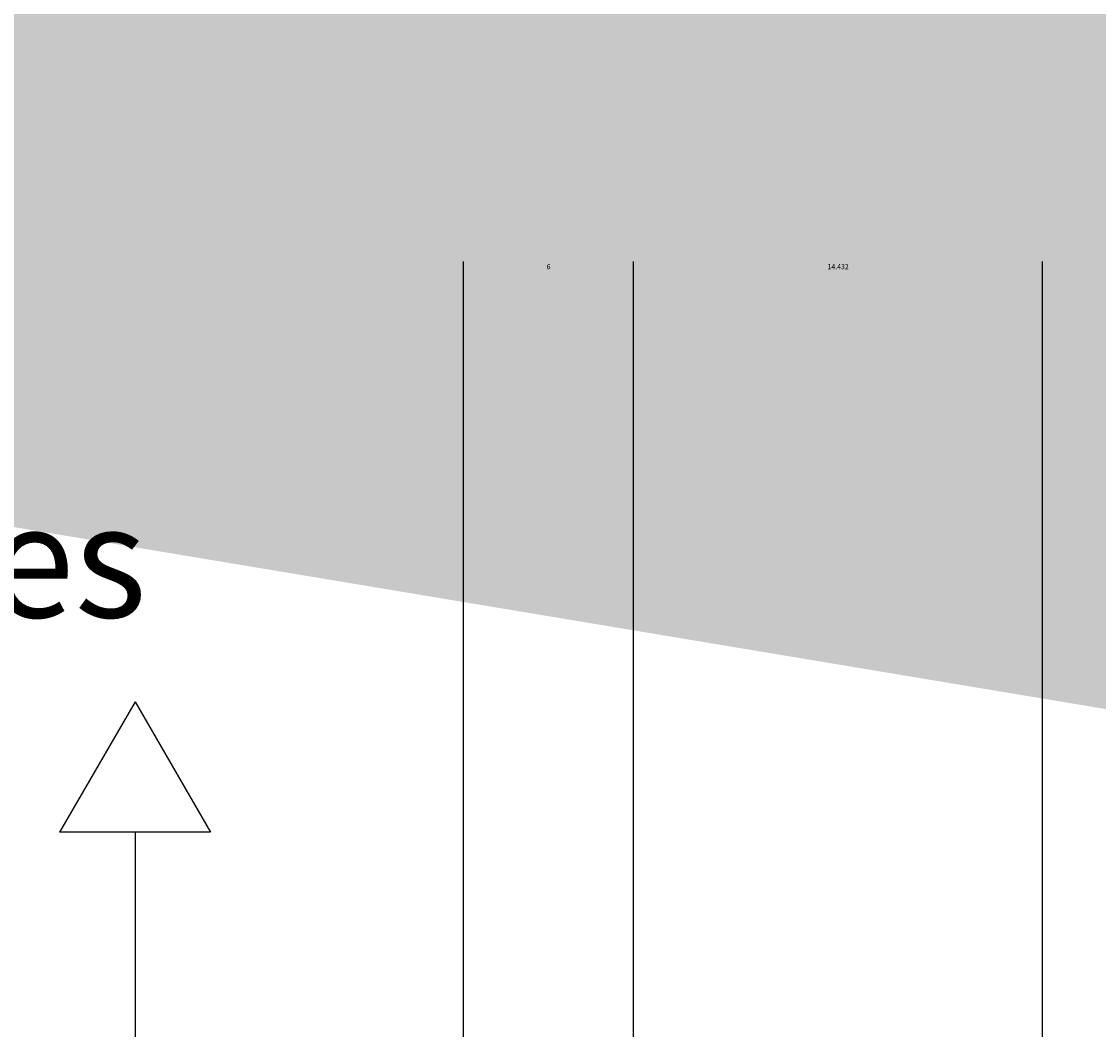
# Model space of a CAD drawing. Units: millimetres. Extents: x -22994 to 29398, y -19990 to 20176.
# Tile 113 of 135: x 166 to 204, y 177 to 213. Entities that reach past the tile are written whole.
import ezdxf

# ---------------------------------------------------------------- set-up
doc = ezdxf.new("R2010")
doc.units = ezdxf.units.MM
doc.header["$MEASUREMENT"] = 0
for name, color, linetype, lineweight in [('M-ANNO-SYMB', 7, 'Continuous', 25), ('M-ANNO-TEXT', 7, 'Continuous', 25), ('M-DIMS', 2, 'Continuous', 18)]:
    doc.layers.add(name, color=color, linetype=linetype, lineweight=lineweight)
doc.styles.get("Standard").update_dxf_attribs({"font": 'arial.ttf'})
doc.dimstyles.get("Standard").update_dxf_attribs({"dimtxt": 0.18, "dimasz": 10000, "dimexe": 0.18, "dimexo": 0.0625, "dimgap": 0.09, "dimtad": 0, "dimtih": 1, "dimtoh": 1, "dimdec": 0, "dimzin": 0, "dimdsep": 46, "dimtxsty": 'Standard', "dimcen": 0.09, "dimadec": 0, "dimazin": 0, "dimtfac": 1, "dimtdec": 0, "dimtofl": 0, "dimtmove": 0, "dimatfit": 3, "dimfxl": 1, "dimtolj": 1, "dimtzin": 0, "dimlwd": 30, "dimarcsym": 0})

# ---------------------------------------------------------------- blocks, each defined once
blk = doc.blocks.new('ARROW-FLOW')
for p, q in [((4.609, 5.322), (0, 2.661)), ((4.609, 5.322), (4.609, 0)), ((4.609, 0), (0, 2.661))]:
    blk.add_line(p, q)
blk = doc.blocks.new('*D2')
at = {"layer": 'Defpoints', "color": 0, "transparency": 16777216}
for p in [(6.677, 10.271), (290.852, 10.271), (290.852, -5.079)]:
    blk.add_point(p, dxfattribs=at)
at = {"layer": 'M-DIMS', "color": 0, "lineweight": -2, "transparency": 16777216}
for p, q in [((6.677, 10.209), (6.677, -5.259)), ((290.852, 10.209), (290.852, -5.259))]:
    blk.add_line(p, q, dxfattribs=at)
at = {"layer": 'M-DIMS', "color": 0, "lineweight": 30, "transparency": 16777216}
for p, q in [((-9993.323, -5.079), (-19993.323, -5.079)), ((10290.852, -5.079), (20290.852, -5.079))]:
    blk.add_line(p, q, dxfattribs=at)
at = {"layer": 'M-DIMS', "color": 0, "transparency": 16777216}
for points in [[(-9993.323, 1661.588), (-9993.323, -1671.745), (6.677, -5.079)], [(10290.852, 1661.588), (10290.852, -1671.745), (290.852, -5.079)]]:
    blk.add_solid(points, dxfattribs=at)
at = {"layer": 'M-DIMS', "color": 0, "transparency": 16777216, "insert": (148.765, -5.079), "char_height": 0.18, "attachment_point": 5}
blk.add_mtext('\\A1;284.2', dxfattribs=at)
blk = doc.blocks.new('*D3')
at = {"layer": 'Defpoints', "color": 0, "transparency": 16777216}
for p in [(110.265, 204.165), (110.265, 176.366), (95.833, 127.967)]:
    blk.add_point(p, dxfattribs=at)
at = {"layer": 'M-DIMS', "color": 0, "lineweight": 30, "transparency": 16777216}
for p, q in [((-9904.167, 204.165), (-19904.167, 204.165)), ((10110.265, 204.165), (20110.265, 204.165))]:
    blk.add_line(p, q, dxfattribs=at)
at = {"layer": 'M-DIMS', "color": 0, "lineweight": -2, "transparency": 16777216}
for p, q in [((95.833, 128.03), (95.833, 204.345)), ((110.265, 176.429), (110.265, 204.345))]:
    blk.add_line(p, q, dxfattribs=at)
at = {"layer": 'M-DIMS', "color": 0, "transparency": 16777216}
for points in [[(-9904.167, 1870.832), (-9904.167, -1462.501), (95.833, 204.165)], [(10110.265, 1870.832), (10110.265, -1462.501), (110.265, 204.165)]]:
    blk.add_solid(points, dxfattribs=at)
at = {"layer": 'M-DIMS', "color": 0, "transparency": 16777216, "insert": (103.049, 204.165), "char_height": 0.18, "attachment_point": 5}
blk.add_mtext('\\A1;14.432', dxfattribs=at)
blk = doc.blocks.new('*D4')
at = {"layer": 'Defpoints', "color": 0, "transparency": 16777216}
for p in [(116.265, 204.165), (110.265, 176.366), (116.265, 176.366)]:
    blk.add_point(p, dxfattribs=at)
at = {"layer": 'M-DIMS', "color": 0, "lineweight": 30, "transparency": 16777216}
for p, q in [((-9889.735, 204.165), (-19889.735, 204.165)), ((10116.265, 204.165), (20116.265, 204.165))]:
    blk.add_line(p, q, dxfattribs=at)
at = {"layer": 'M-DIMS', "color": 0, "lineweight": -2, "transparency": 16777216}
for p, q in [((110.265, 176.429), (110.265, 204.345)), ((116.265, 176.429), (116.265, 204.345))]:
    blk.add_line(p, q, dxfattribs=at)
at = {"layer": 'M-DIMS', "color": 0, "transparency": 16777216}
for points in [[(-9889.735, 1870.832), (-9889.735, -1462.501), (110.265, 204.165)], [(10116.265, 1870.832), (10116.265, -1462.501), (116.265, 204.165)]]:
    blk.add_solid(points, dxfattribs=at)
at = {"layer": 'M-DIMS', "color": 0, "transparency": 16777216, "insert": (113.265, 204.165), "char_height": 0.18, "attachment_point": 5}
blk.add_mtext('\\A1;6', dxfattribs=at)
blk = doc.blocks.new('*D5')
at = {"layer": 'Defpoints', "color": 0, "transparency": 16777216}
for p in [(181.265, 204.165), (116.265, 176.366), (181.265, 176.366)]:
    blk.add_point(p, dxfattribs=at)
at = {"layer": 'M-DIMS', "color": 0, "lineweight": 30, "transparency": 16777216}
for p, q in [((-9883.735, 204.165), (-19883.735, 204.165)), ((10181.265, 204.165), (20181.265, 204.165))]:
    blk.add_line(p, q, dxfattribs=at)
at = {"layer": 'M-DIMS', "color": 0, "lineweight": -2, "transparency": 16777216}
for p, q in [((116.265, 176.429), (116.265, 204.345)), ((181.265, 176.429), (181.265, 204.345))]:
    blk.add_line(p, q, dxfattribs=at)
at = {"layer": 'M-DIMS', "color": 0, "transparency": 16777216}
for points in [[(-9883.735, 1870.832), (-9883.735, -1462.501), (116.265, 204.165)], [(10181.265, 1870.832), (10181.265, -1462.501), (181.265, 204.165)]]:
    blk.add_solid(points, dxfattribs=at)
at = {"layer": 'M-DIMS', "color": 0, "transparency": 16777216, "insert": (148.765, 204.165), "char_height": 0.18, "attachment_point": 5}
blk.add_mtext('\\A1;65', dxfattribs=at)
blk = doc.blocks.new('*D6')
at = {"layer": 'Defpoints', "color": 0, "transparency": 16777216}
for p in [(187.265, 204.165), (181.265, 176.366), (187.265, 176.366)]:
    blk.add_point(p, dxfattribs=at)
at = {"layer": 'M-DIMS', "color": 0, "lineweight": 30, "transparency": 16777216}
for p, q in [((-9818.735, 204.165), (-19818.735, 204.165)), ((10187.265, 204.165), (20187.265, 204.165))]:
    blk.add_line(p, q, dxfattribs=at)
at = {"layer": 'M-DIMS', "color": 0, "lineweight": -2, "transparency": 16777216}
for p, q in [((181.265, 176.429), (181.265, 204.345)), ((187.265, 176.429), (187.265, 204.345))]:
    blk.add_line(p, q, dxfattribs=at)
at = {"layer": 'M-DIMS', "color": 0, "transparency": 16777216}
for points in [[(-9818.735, 1870.832), (-9818.735, -1462.501), (181.265, 204.165)], [(10187.265, 1870.832), (10187.265, -1462.501), (187.265, 204.165)]]:
    blk.add_solid(points, dxfattribs=at)
at = {"layer": 'M-DIMS', "color": 0, "transparency": 16777216, "insert": (184.265, 204.165), "char_height": 0.18, "attachment_point": 5}
blk.add_mtext('\\A1;6', dxfattribs=at)
blk = doc.blocks.new('*D7')
at = {"layer": 'Defpoints', "color": 0, "transparency": 16777216}
for p in [(201.697, 204.165), (187.265, 176.366), (201.697, 127.967)]:
    blk.add_point(p, dxfattribs=at)
at = {"layer": 'M-DIMS', "color": 0, "lineweight": 30, "transparency": 16777216}
for p, q in [((-9812.735, 204.165), (-19812.735, 204.165)), ((10201.697, 204.165), (20201.697, 204.165))]:
    blk.add_line(p, q, dxfattribs=at)
at = {"layer": 'M-DIMS', "color": 0, "lineweight": -2, "transparency": 16777216}
for p, q in [((187.265, 176.429), (187.265, 204.345)), ((201.697, 128.03), (201.697, 204.345))]:
    blk.add_line(p, q, dxfattribs=at)
at = {"layer": 'M-DIMS', "color": 0, "transparency": 16777216}
for points in [[(-9812.735, 1870.832), (-9812.735, -1462.501), (187.265, 204.165)], [(10201.697, 1870.832), (10201.697, -1462.501), (201.697, 204.165)]]:
    blk.add_solid(points, dxfattribs=at)
at = {"layer": 'M-DIMS', "color": 0, "transparency": 16777216, "insert": (194.481, 204.165), "char_height": 0.18, "attachment_point": 5}
blk.add_mtext('\\A1;14.432', dxfattribs=at)
blk = doc.blocks.new('*D8')
at = {"layer": 'Defpoints', "color": 0, "transparency": 16777216}
for p in [(227.648, 204.165), (227.648, 146.73), (201.697, 127.967)]:
    blk.add_point(p, dxfattribs=at)
at = {"layer": 'M-DIMS', "color": 0, "lineweight": 30, "transparency": 16777216}
for p, q in [((-9798.303, 204.165), (-19798.303, 204.165)), ((10227.648, 204.165), (20227.648, 204.165))]:
    blk.add_line(p, q, dxfattribs=at)
at = {"layer": 'M-DIMS', "color": 0, "lineweight": -2, "transparency": 16777216}
for p, q in [((201.697, 128.03), (201.697, 204.345)), ((227.648, 146.792), (227.648, 204.345))]:
    blk.add_line(p, q, dxfattribs=at)
at = {"layer": 'M-DIMS', "color": 0, "transparency": 16777216}
for points in [[(-9798.303, 1870.832), (-9798.303, -1462.501), (201.697, 204.165)], [(10227.648, 1870.832), (10227.648, -1462.501), (227.648, 204.165)]]:
    blk.add_solid(points, dxfattribs=at)
at = {"layer": 'M-DIMS', "color": 0, "transparency": 16777216, "insert": (214.673, 204.165), "char_height": 0.18, "attachment_point": 5}
blk.add_mtext('\\A1;25.95', dxfattribs=at)
blk = doc.blocks.new('*D9')
at = {"layer": 'Defpoints', "color": 0, "transparency": 16777216}
for p in [(187.265, 176.366), (306.202, 176.366), (290.852, 10.271)]:
    blk.add_point(p, dxfattribs=at)
at = {"layer": 'M-DIMS', "color": 0, "lineweight": 30, "transparency": 16777216}
for p, q in [((306.202, 10176.366), (306.202, 20176.366)), ((306.202, -9989.729), (306.202, -19989.729))]:
    blk.add_line(p, q, dxfattribs=at)
at = {"layer": 'M-DIMS', "color": 0, "lineweight": -2, "transparency": 16777216}
for p, q in [((187.327, 176.366), (306.382, 176.366)), ((290.915, 10.271), (306.382, 10.271))]:
    blk.add_line(p, q, dxfattribs=at)
at = {"layer": 'M-DIMS', "color": 0, "transparency": 16777216}
for points in [[(-1360.465, 10176.366), (1972.869, 10176.366), (306.202, 176.366)], [(-1360.465, -9989.729), (1972.869, -9989.729), (306.202, 10.271)]]:
    blk.add_solid(points, dxfattribs=at)
at = {"layer": 'M-DIMS', "color": 0, "transparency": 16777216, "insert": (306.202, 93.319), "char_height": 0.18, "attachment_point": 5}
blk.add_mtext('\\A1;166.1', dxfattribs=at)
blk = doc.blocks.new('*D10')
at = {"layer": 'Defpoints', "color": 0, "transparency": 16777216}
for p in [(125.65, 136.071), (133.346, 136.071), (133.346, -5.079)]:
    blk.add_point(p, dxfattribs=at)
at = {"layer": 'M-DIMS', "color": 0, "lineweight": -2, "transparency": 16777216}
for p, q in [((125.65, 136.009), (125.65, -5.259)), ((133.346, 136.009), (133.346, -5.259))]:
    blk.add_line(p, q, dxfattribs=at)
at = {"layer": 'M-DIMS', "color": 0, "lineweight": 30, "transparency": 16777216}
for p, q in [((-9874.35, -5.079), (-19874.35, -5.079)), ((10133.346, -5.079), (20133.346, -5.079))]:
    blk.add_line(p, q, dxfattribs=at)
at = {"layer": 'M-DIMS', "color": 0, "transparency": 16777216}
for points in [[(-9874.35, 1661.588), (-9874.35, -1671.745), (125.65, -5.079)], [(10133.346, 1661.588), (10133.346, -1671.745), (133.346, -5.079)]]:
    blk.add_solid(points, dxfattribs=at)
at = {"layer": 'M-DIMS', "color": 0, "transparency": 16777216, "insert": (129.498, -5.079), "char_height": 0.18, "attachment_point": 5}
blk.add_mtext('\\A1;7.696', dxfattribs=at)
blk = doc.blocks.new('*D11')
at = {"layer": 'Defpoints', "color": 0, "transparency": 16777216}
for p in [(133.346, 136.071), (135.65, 136.071), (135.65, -5.079)]:
    blk.add_point(p, dxfattribs=at)
at = {"layer": 'M-DIMS', "color": 0, "lineweight": -2, "transparency": 16777216}
for p, q in [((133.346, 136.009), (133.346, -5.259)), ((135.65, 136.009), (135.65, -5.259))]:
    blk.add_line(p, q, dxfattribs=at)
at = {"layer": 'M-DIMS', "color": 0, "lineweight": 30, "transparency": 16777216}
for p, q in [((-9866.654, -5.079), (-19866.654, -5.079)), ((10135.65, -5.079), (20135.65, -5.079))]:
    blk.add_line(p, q, dxfattribs=at)
at = {"layer": 'M-DIMS', "color": 0, "transparency": 16777216}
for points in [[(-9866.654, 1661.588), (-9866.654, -1671.745), (133.346, -5.079)], [(10135.65, 1661.588), (10135.65, -1671.745), (135.65, -5.079)]]:
    blk.add_solid(points, dxfattribs=at)
at = {"layer": 'M-DIMS', "color": 0, "transparency": 16777216, "insert": (134.498, -5.079), "char_height": 0.18, "attachment_point": 5}
blk.add_mtext('\\A1;2.304', dxfattribs=at)
blk = doc.blocks.new('*D12')
at = {"layer": 'Defpoints', "color": 0, "transparency": 16777216}
for p in [(135.65, 136.071), (145.65, 136.071), (145.65, -5.079)]:
    blk.add_point(p, dxfattribs=at)
at = {"layer": 'M-DIMS', "color": 0, "lineweight": -2, "transparency": 16777216}
for p, q in [((135.65, 136.009), (135.65, -5.259)), ((145.65, 136.009), (145.65, -5.259))]:
    blk.add_line(p, q, dxfattribs=at)
at = {"layer": 'M-DIMS', "color": 0, "lineweight": 30, "transparency": 16777216}
for p, q in [((-9864.35, -5.079), (-19864.35, -5.079)), ((10145.65, -5.079), (20145.65, -5.079))]:
    blk.add_line(p, q, dxfattribs=at)
at = {"layer": 'M-DIMS', "color": 0, "transparency": 16777216}
for points in [[(-9864.35, 1661.588), (-9864.35, -1671.745), (135.65, -5.079)], [(10145.65, 1661.588), (10145.65, -1671.745), (145.65, -5.079)]]:
    blk.add_solid(points, dxfattribs=at)
at = {"layer": 'M-DIMS', "color": 0, "transparency": 16777216, "insert": (140.65, -5.079), "char_height": 0.18, "attachment_point": 5}
blk.add_mtext('\\A1;10', dxfattribs=at)
blk = doc.blocks.new('*D13')
at = {"layer": 'Defpoints', "color": 0, "transparency": 16777216}
for p in [(145.65, 136.071), (155.65, 136.071), (155.65, -5.079)]:
    blk.add_point(p, dxfattribs=at)
at = {"layer": 'M-DIMS', "color": 0, "lineweight": -2, "transparency": 16777216}
for p, q in [((145.65, 136.009), (145.65, -5.259)), ((155.65, 136.009), (155.65, -5.259))]:
    blk.add_line(p, q, dxfattribs=at)
at = {"layer": 'M-DIMS', "color": 0, "lineweight": 30, "transparency": 16777216}
for p, q in [((-9854.35, -5.079), (-19854.35, -5.079)), ((10155.65, -5.079), (20155.65, -5.079))]:
    blk.add_line(p, q, dxfattribs=at)
at = {"layer": 'M-DIMS', "color": 0, "transparency": 16777216}
for points in [[(-9854.35, 1661.588), (-9854.35, -1671.745), (145.65, -5.079)], [(10155.65, 1661.588), (10155.65, -1671.745), (155.65, -5.079)]]:
    blk.add_solid(points, dxfattribs=at)
at = {"layer": 'M-DIMS', "color": 0, "transparency": 16777216, "insert": (150.65, -5.079), "char_height": 0.18, "attachment_point": 5}
blk.add_mtext('\\A1;10', dxfattribs=at)
blk = doc.blocks.new('*D14')
at = {"layer": 'Defpoints', "color": 0, "transparency": 16777216}
for p in [(155.65, 136.071), (165.65, 136.071), (165.65, -5.079)]:
    blk.add_point(p, dxfattribs=at)
at = {"layer": 'M-DIMS', "color": 0, "lineweight": -2, "transparency": 16777216}
for p, q in [((155.65, 136.009), (155.65, -5.259)), ((165.65, 136.009), (165.65, -5.259))]:
    blk.add_line(p, q, dxfattribs=at)
at = {"layer": 'M-DIMS', "color": 0, "lineweight": 30, "transparency": 16777216}
for p, q in [((-9844.35, -5.079), (-19844.35, -5.079)), ((10165.65, -5.079), (20165.65, -5.079))]:
    blk.add_line(p, q, dxfattribs=at)
at = {"layer": 'M-DIMS', "color": 0, "transparency": 16777216}
for points in [[(-9844.35, 1661.588), (-9844.35, -1671.745), (155.65, -5.079)], [(10165.65, 1661.588), (10165.65, -1671.745), (165.65, -5.079)]]:
    blk.add_solid(points, dxfattribs=at)
at = {"layer": 'M-DIMS', "color": 0, "transparency": 16777216, "insert": (160.65, -5.079), "char_height": 0.18, "attachment_point": 5}
blk.add_mtext('\\A1;10', dxfattribs=at)
blk = doc.blocks.new('*D15')
at = {"layer": 'Defpoints', "color": 0, "transparency": 16777216}
for p in [(173.346, 154.788), (173.346, 136.071), (306.202, 136.071)]:
    blk.add_point(p, dxfattribs=at)
at = {"layer": 'M-DIMS', "color": 0, "lineweight": 30, "transparency": 16777216}
for p, q in [((306.202, 10154.788), (306.202, 20154.788)), ((306.202, -9863.929), (306.202, -19863.929))]:
    blk.add_line(p, q, dxfattribs=at)
at = {"layer": 'M-DIMS', "color": 0, "lineweight": -2, "transparency": 16777216}
for p, q in [((173.408, 154.788), (306.382, 154.788)), ((173.408, 136.071), (306.382, 136.071))]:
    blk.add_line(p, q, dxfattribs=at)
at = {"layer": 'M-DIMS', "color": 0, "transparency": 16777216}
for points in [[(-1360.465, 10154.788), (1972.869, 10154.788), (306.202, 154.788)], [(-1360.465, -9863.929), (1972.869, -9863.929), (306.202, 136.071)]]:
    blk.add_solid(points, dxfattribs=at)
at = {"layer": 'M-DIMS', "color": 0, "transparency": 16777216, "insert": (306.202, 145.43), "char_height": 0.18, "attachment_point": 5}
blk.add_mtext('\\A1;18.717', dxfattribs=at)
blk = doc.blocks.new('*D16')
at = {"layer": 'Defpoints', "color": 0, "transparency": 16777216}
for p in [(120.17, 204.165), (110.466, 48.035), (120.17, 48.035)]:
    blk.add_point(p, dxfattribs=at)
at = {"layer": 'M-DIMS', "color": 0, "lineweight": 30, "transparency": 16777216}
for p, q in [((-9889.534, 204.165), (-19889.534, 204.165)), ((10120.17, 204.165), (20120.17, 204.165))]:
    blk.add_line(p, q, dxfattribs=at)
at = {"layer": 'M-DIMS', "color": 0, "lineweight": -2, "transparency": 16777216}
for p, q in [((110.466, 48.097), (110.466, 204.345)), ((120.17, 48.097), (120.17, 204.345))]:
    blk.add_line(p, q, dxfattribs=at)
at = {"layer": 'M-DIMS', "color": 0, "transparency": 16777216}
for points in [[(-9889.534, 1870.832), (-9889.534, -1462.501), (110.466, 204.165)], [(10120.17, 1870.832), (10120.17, -1462.501), (120.17, 204.165)]]:
    blk.add_solid(points, dxfattribs=at)
at = {"layer": 'M-DIMS', "color": 0, "transparency": 16777216, "insert": (115.318, 204.165), "char_height": 0.18, "attachment_point": 5}
blk.add_mtext('\\A1;9.704', dxfattribs=at)
blk = doc.blocks.new('*D17')
at = {"layer": 'Defpoints', "color": 0, "transparency": 16777216}
for p in [(126.17, 204.165), (120.17, 48.035), (126.17, 48.035)]:
    blk.add_point(p, dxfattribs=at)
at = {"layer": 'M-DIMS', "color": 0, "lineweight": 30, "transparency": 16777216}
for p, q in [((-9879.83, 204.165), (-19879.83, 204.165)), ((10126.17, 204.165), (20126.17, 204.165))]:
    blk.add_line(p, q, dxfattribs=at)
at = {"layer": 'M-DIMS', "color": 0, "lineweight": -2, "transparency": 16777216}
for p, q in [((120.17, 48.097), (120.17, 204.345)), ((126.17, 48.097), (126.17, 204.345))]:
    blk.add_line(p, q, dxfattribs=at)
at = {"layer": 'M-DIMS', "color": 0, "transparency": 16777216}
for points in [[(-9879.83, 1870.832), (-9879.83, -1462.501), (120.17, 204.165)], [(10126.17, 1870.832), (10126.17, -1462.501), (126.17, 204.165)]]:
    blk.add_solid(points, dxfattribs=at)
at = {"layer": 'M-DIMS', "color": 0, "transparency": 16777216, "insert": (123.17, 204.165), "char_height": 0.18, "attachment_point": 5}
blk.add_mtext('\\A1;6', dxfattribs=at)
blk = doc.blocks.new('*D18')
at = {"layer": 'Defpoints', "color": 0, "transparency": 16777216}
for p in [(132.17, 204.165), (126.17, 48.035), (132.17, 48.035)]:
    blk.add_point(p, dxfattribs=at)
at = {"layer": 'M-DIMS', "color": 0, "lineweight": 30, "transparency": 16777216}
for p, q in [((-9873.83, 204.165), (-19873.83, 204.165)), ((10132.17, 204.165), (20132.17, 204.165))]:
    blk.add_line(p, q, dxfattribs=at)
at = {"layer": 'M-DIMS', "color": 0, "lineweight": -2, "transparency": 16777216}
for p, q in [((126.17, 48.097), (126.17, 204.345)), ((132.17, 48.097), (132.17, 204.345))]:
    blk.add_line(p, q, dxfattribs=at)
at = {"layer": 'M-DIMS', "color": 0, "transparency": 16777216}
for points in [[(-9873.83, 1870.832), (-9873.83, -1462.501), (126.17, 204.165)], [(10132.17, 1870.832), (10132.17, -1462.501), (132.17, 204.165)]]:
    blk.add_solid(points, dxfattribs=at)
at = {"layer": 'M-DIMS', "color": 0, "transparency": 16777216, "insert": (129.17, 204.165), "char_height": 0.18, "attachment_point": 5}
blk.add_mtext('\\A1;6', dxfattribs=at)
blk = doc.blocks.new('*D19')
at = {"layer": 'Defpoints', "color": 0, "transparency": 16777216}
for p in [(138.17, 204.165), (132.17, 48.035), (138.17, 48.035)]:
    blk.add_point(p, dxfattribs=at)
at = {"layer": 'M-DIMS', "color": 0, "lineweight": 30, "transparency": 16777216}
for p, q in [((-9867.83, 204.165), (-19867.83, 204.165)), ((10138.17, 204.165), (20138.17, 204.165))]:
    blk.add_line(p, q, dxfattribs=at)
at = {"layer": 'M-DIMS', "color": 0, "lineweight": -2, "transparency": 16777216}
for p, q in [((132.17, 48.097), (132.17, 204.345)), ((138.17, 48.097), (138.17, 204.345))]:
    blk.add_line(p, q, dxfattribs=at)
at = {"layer": 'M-DIMS', "color": 0, "transparency": 16777216}
for points in [[(-9867.83, 1870.832), (-9867.83, -1462.501), (132.17, 204.165)], [(10138.17, 1870.832), (10138.17, -1462.501), (138.17, 204.165)]]:
    blk.add_solid(points, dxfattribs=at)
at = {"layer": 'M-DIMS', "color": 0, "transparency": 16777216, "insert": (135.17, 204.165), "char_height": 0.18, "attachment_point": 5}
blk.add_mtext('\\A1;6', dxfattribs=at)
blk = doc.blocks.new('*D20')
at = {"layer": 'Defpoints', "color": 0, "transparency": 16777216}
for p in [(144.17, 204.165), (138.17, 48.035), (144.17, 48.035)]:
    blk.add_point(p, dxfattribs=at)
at = {"layer": 'M-DIMS', "color": 0, "lineweight": 30, "transparency": 16777216}
for p, q in [((-9861.83, 204.165), (-19861.83, 204.165)), ((10144.17, 204.165), (20144.17, 204.165))]:
    blk.add_line(p, q, dxfattribs=at)
at = {"layer": 'M-DIMS', "color": 0, "lineweight": -2, "transparency": 16777216}
for p, q in [((138.17, 48.097), (138.17, 204.345)), ((144.17, 48.097), (144.17, 204.345))]:
    blk.add_line(p, q, dxfattribs=at)
at = {"layer": 'M-DIMS', "color": 0, "transparency": 16777216}
for points in [[(-9861.83, 1870.832), (-9861.83, -1462.501), (138.17, 204.165)], [(10144.17, 1870.832), (10144.17, -1462.501), (144.17, 204.165)]]:
    blk.add_solid(points, dxfattribs=at)
at = {"layer": 'M-DIMS', "color": 0, "transparency": 16777216, "insert": (141.17, 204.165), "char_height": 0.18, "attachment_point": 5}
blk.add_mtext('\\A1;6', dxfattribs=at)
blk = doc.blocks.new('*D21')
at = {"layer": 'Defpoints', "color": 0, "transparency": 16777216}
for p in [(149.116, 204.165), (144.17, 48.035), (149.116, 48.035)]:
    blk.add_point(p, dxfattribs=at)
at = {"layer": 'M-DIMS', "color": 0, "lineweight": 30, "transparency": 16777216}
for p, q in [((-9855.83, 204.165), (-19855.83, 204.165)), ((10149.116, 204.165), (20149.116, 204.165))]:
    blk.add_line(p, q, dxfattribs=at)
at = {"layer": 'M-DIMS', "color": 0, "lineweight": -2, "transparency": 16777216}
for p, q in [((144.17, 48.097), (144.17, 204.345)), ((149.116, 48.097), (149.116, 204.345))]:
    blk.add_line(p, q, dxfattribs=at)
at = {"layer": 'M-DIMS', "color": 0, "transparency": 16777216}
for points in [[(-9855.83, 1870.832), (-9855.83, -1462.501), (144.17, 204.165)], [(10149.116, 1870.832), (10149.116, -1462.501), (149.116, 204.165)]]:
    blk.add_solid(points, dxfattribs=at)
at = {"layer": 'M-DIMS', "color": 0, "transparency": 16777216, "insert": (146.643, 204.165), "char_height": 0.18, "attachment_point": 5}
blk.add_mtext('\\A1;4.945', dxfattribs=at)
blk = doc.blocks.new('*D22')
at = {"layer": 'Defpoints', "color": 0, "transparency": 16777216}
for p in [(149.116, 30.99), (155.116, 30.99), (155.116, -5.079)]:
    blk.add_point(p, dxfattribs=at)
at = {"layer": 'M-DIMS', "color": 0, "lineweight": -2, "transparency": 16777216}
for p, q in [((149.116, 30.927), (149.116, -5.259)), ((155.116, 30.927), (155.116, -5.259))]:
    blk.add_line(p, q, dxfattribs=at)
at = {"layer": 'M-DIMS', "color": 0, "lineweight": 30, "transparency": 16777216}
for p, q in [((-9850.884, -5.079), (-19850.884, -5.079)), ((10155.116, -5.079), (20155.116, -5.079))]:
    blk.add_line(p, q, dxfattribs=at)
at = {"layer": 'M-DIMS', "color": 0, "transparency": 16777216}
for points in [[(-9850.884, 1661.588), (-9850.884, -1671.745), (149.116, -5.079)], [(10155.116, 1661.588), (10155.116, -1671.745), (155.116, -5.079)]]:
    blk.add_solid(points, dxfattribs=at)
at = {"layer": 'M-DIMS', "color": 0, "transparency": 16777216, "insert": (152.116, -5.079), "char_height": 0.18, "attachment_point": 5}
blk.add_mtext('\\A1;6', dxfattribs=at)
blk = doc.blocks.new('*D23')
at = {"layer": 'Defpoints', "color": 0, "transparency": 16777216}
for p in [(155.116, 30.99), (161.116, 30.99), (161.116, -5.079)]:
    blk.add_point(p, dxfattribs=at)
at = {"layer": 'M-DIMS', "color": 0, "lineweight": -2, "transparency": 16777216}
for p, q in [((155.116, 30.927), (155.116, -5.259)), ((161.116, 30.927), (161.116, -5.259))]:
    blk.add_line(p, q, dxfattribs=at)
at = {"layer": 'M-DIMS', "color": 0, "lineweight": 30, "transparency": 16777216}
for p, q in [((-9844.884, -5.079), (-19844.884, -5.079)), ((10161.116, -5.079), (20161.116, -5.079))]:
    blk.add_line(p, q, dxfattribs=at)
at = {"layer": 'M-DIMS', "color": 0, "transparency": 16777216}
for points in [[(-9844.884, 1661.588), (-9844.884, -1671.745), (155.116, -5.079)], [(10161.116, 1661.588), (10161.116, -1671.745), (161.116, -5.079)]]:
    blk.add_solid(points, dxfattribs=at)
at = {"layer": 'M-DIMS', "color": 0, "transparency": 16777216, "insert": (158.116, -5.079), "char_height": 0.18, "attachment_point": 5}
blk.add_mtext('\\A1;6', dxfattribs=at)
blk = doc.blocks.new('*D24')
at = {"layer": 'Defpoints', "color": 0, "transparency": 16777216}
for p in [(161.116, 30.99), (166.439, 30.99), (166.439, -5.079)]:
    blk.add_point(p, dxfattribs=at)
at = {"layer": 'M-DIMS', "color": 0, "lineweight": -2, "transparency": 16777216}
for p, q in [((161.116, 30.927), (161.116, -5.259)), ((166.439, 30.927), (166.439, -5.259))]:
    blk.add_line(p, q, dxfattribs=at)
at = {"layer": 'M-DIMS', "color": 0, "lineweight": 30, "transparency": 16777216}
for p, q in [((-9838.884, -5.079), (-19838.884, -5.079)), ((10166.439, -5.079), (20166.439, -5.079))]:
    blk.add_line(p, q, dxfattribs=at)
at = {"layer": 'M-DIMS', "color": 0, "transparency": 16777216}
for points in [[(-9838.884, 1661.588), (-9838.884, -1671.745), (161.116, -5.079)], [(10166.439, 1661.588), (10166.439, -1671.745), (166.439, -5.079)]]:
    blk.add_solid(points, dxfattribs=at)
at = {"layer": 'M-DIMS', "color": 0, "transparency": 16777216, "insert": (163.777, -5.079), "char_height": 0.18, "attachment_point": 5}
blk.add_mtext('\\A1;5.323', dxfattribs=at)
blk = doc.blocks.new('*D25')
at = {"layer": 'Defpoints', "color": 0, "transparency": 16777216}
for p in [(166.439, 30.99), (172.439, 30.99), (172.439, -5.079)]:
    blk.add_point(p, dxfattribs=at)
at = {"layer": 'M-DIMS', "color": 0, "lineweight": -2, "transparency": 16777216}
for p, q in [((166.439, 30.927), (166.439, -5.259)), ((172.439, 30.927), (172.439, -5.259))]:
    blk.add_line(p, q, dxfattribs=at)
at = {"layer": 'M-DIMS', "color": 0, "lineweight": 30, "transparency": 16777216}
for p, q in [((-9833.561, -5.079), (-19833.561, -5.079)), ((10172.439, -5.079), (20172.439, -5.079))]:
    blk.add_line(p, q, dxfattribs=at)
at = {"layer": 'M-DIMS', "color": 0, "transparency": 16777216}
for points in [[(-9833.561, 1661.588), (-9833.561, -1671.745), (166.439, -5.079)], [(10172.439, 1661.588), (10172.439, -1671.745), (172.439, -5.079)]]:
    blk.add_solid(points, dxfattribs=at)
at = {"layer": 'M-DIMS', "color": 0, "transparency": 16777216, "insert": (169.439, -5.079), "char_height": 0.18, "attachment_point": 5}
blk.add_mtext('\\A1;6', dxfattribs=at)
blk = doc.blocks.new('*D26')
at = {"layer": 'Defpoints', "color": 0, "transparency": 16777216}
for p in [(172.439, 30.99), (178.439, 30.99), (178.439, -5.079)]:
    blk.add_point(p, dxfattribs=at)
at = {"layer": 'M-DIMS', "color": 0, "lineweight": -2, "transparency": 16777216}
for p, q in [((172.439, 30.927), (172.439, -5.259)), ((178.439, 30.927), (178.439, -5.259))]:
    blk.add_line(p, q, dxfattribs=at)
at = {"layer": 'M-DIMS', "color": 0, "lineweight": 30, "transparency": 16777216}
for p, q in [((-9827.561, -5.079), (-19827.561, -5.079)), ((10178.439, -5.079), (20178.439, -5.079))]:
    blk.add_line(p, q, dxfattribs=at)
at = {"layer": 'M-DIMS', "color": 0, "transparency": 16777216}
for points in [[(-9827.561, 1661.588), (-9827.561, -1671.745), (172.439, -5.079)], [(10178.439, 1661.588), (10178.439, -1671.745), (178.439, -5.079)]]:
    blk.add_solid(points, dxfattribs=at)
at = {"layer": 'M-DIMS', "color": 0, "transparency": 16777216, "insert": (175.439, -5.079), "char_height": 0.18, "attachment_point": 5}
blk.add_mtext('\\A1;6', dxfattribs=at)
blk = doc.blocks.new('*D27')
at = {"layer": 'Defpoints', "color": 0, "transparency": 16777216}
for p in [(178.439, 30.99), (188.117, 30.99), (188.117, -5.079)]:
    blk.add_point(p, dxfattribs=at)
at = {"layer": 'M-DIMS', "color": 0, "lineweight": -2, "transparency": 16777216}
for p, q in [((178.439, 30.927), (178.439, -5.259)), ((188.117, 30.927), (188.117, -5.259))]:
    blk.add_line(p, q, dxfattribs=at)
at = {"layer": 'M-DIMS', "color": 0, "lineweight": 30, "transparency": 16777216}
for p, q in [((-9821.561, -5.079), (-19821.561, -5.079)), ((10188.117, -5.079), (20188.117, -5.079))]:
    blk.add_line(p, q, dxfattribs=at)
at = {"layer": 'M-DIMS', "color": 0, "transparency": 16777216}
for points in [[(-9821.561, 1661.588), (-9821.561, -1671.745), (178.439, -5.079)], [(10188.117, 1661.588), (10188.117, -1671.745), (188.117, -5.079)]]:
    blk.add_solid(points, dxfattribs=at)
at = {"layer": 'M-DIMS', "color": 0, "transparency": 16777216, "insert": (183.278, -5.079), "char_height": 0.18, "attachment_point": 5}
blk.add_mtext('\\A1;9.679', dxfattribs=at)
blk = doc.blocks.new('*D28')
at = {"layer": 'Defpoints', "color": 0, "transparency": 16777216}
for p in [(188.117, 48.035), (306.202, 48.035), (188.117, 30.99)]:
    blk.add_point(p, dxfattribs=at)
at = {"layer": 'M-DIMS', "color": 0, "lineweight": 30, "transparency": 16777216}
for p, q in [((306.202, 10048.035), (306.202, 20048.035)), ((306.202, -9969.01), (306.202, -19969.01))]:
    blk.add_line(p, q, dxfattribs=at)
at = {"layer": 'M-DIMS', "color": 0, "lineweight": -2, "transparency": 16777216}
for p, q in [((188.18, 48.035), (306.382, 48.035)), ((188.18, 30.99), (306.382, 30.99))]:
    blk.add_line(p, q, dxfattribs=at)
at = {"layer": 'M-DIMS', "color": 0, "transparency": 16777216}
for points in [[(-1360.465, 10048.035), (1972.869, 10048.035), (306.202, 48.035)], [(-1360.465, -9969.01), (1972.869, -9969.01), (306.202, 30.99)]]:
    blk.add_solid(points, dxfattribs=at)
at = {"layer": 'M-DIMS', "color": 0, "transparency": 16777216, "insert": (306.202, 39.512), "char_height": 0.18, "attachment_point": 5}
blk.add_mtext('\\A1;17.045', dxfattribs=at)
blk = doc.blocks.new('*D29')
at = {"layer": 'Defpoints', "color": 0, "transparency": 16777216}
for p in [(36.801, 80.045), (64.03, 80.045)]:
    blk.add_point(p, dxfattribs=at)
at = {"layer": 'M-DIMS', "color": 0, "lineweight": -2, "transparency": 16777216}
for p, q in [((50.325, 80.045), (50.505, 80.045)), ((50.415, 79.955), (50.415, 80.135))]:
    blk.add_line(p, q, dxfattribs=at)
at = {"layer": 'M-DIMS', "color": 0, "lineweight": 30, "transparency": 16777216}
blk.add_line((20064.03, 80.03), (10064.03, 80.038), dxfattribs=at)
at = {"layer": 'M-DIMS', "color": 0, "transparency": 16777216}
blk.add_solid([(10064.031, 1746.704), (10064.028, -1586.629), (64.03, 80.045)], dxfattribs=at)
at = {"layer": 'M-DIMS', "color": 0, "transparency": 16777216, "insert": (20064.521, 80.03), "char_height": 0.18, "attachment_point": 5}
blk.add_mtext('\\A1;∅27.23', dxfattribs=at)
blk = doc.blocks.new('*D34')
at = {"layer": 'Defpoints', "color": 0, "transparency": 16777216}
for p in [(178.58, 122.895), (176.812, 121.128)]:
    blk.add_point(p, dxfattribs=at)
at = {"layer": 'M-DIMS', "color": 0, "lineweight": 30, "transparency": 16777216}
for p, q in [((14322.436, 14263.311), (7250.508, 7193.103)), ((24322.436, 14263.311), (14322.436, 14263.311))]:
    blk.add_line(p, q, dxfattribs=at)
at = {"layer": 'M-DIMS', "color": 0, "lineweight": -2, "transparency": 16777216}
for p, q in [((176.722, 121.128), (176.902, 121.128)), ((176.812, 121.038), (176.812, 121.218))]:
    blk.add_line(p, q, dxfattribs=at)
at = {"layer": 'M-DIMS', "color": 0, "transparency": 16777216}
blk.add_solid([(6072.14, 8371.758), (8428.876, 6014.448), (178.58, 122.895)], dxfattribs=at)
at = {"layer": 'M-DIMS', "color": 0, "transparency": 16777216, "insert": (24322.97, 14263.311), "char_height": 0.18, "attachment_point": 5}
blk.add_mtext('\\A1;6X R2.5', dxfattribs=at)
blk = doc.blocks.new('*D36')
at = {"layer": 'Defpoints', "color": 0, "transparency": 16777216}
for p in [(46.39, 31.303), (46.387, 26.593)]:
    blk.add_point(p, dxfattribs=at)
at = {"layer": 'M-DIMS', "color": 0, "lineweight": 30, "transparency": 16777216}
for p, q in [((57.15, 20031.301), (51.77, 10031.302)), ((10057.15, 20031.301), (57.15, 20031.301))]:
    blk.add_line(p, q, dxfattribs=at)
at = {"layer": 'M-DIMS', "color": 0, "lineweight": -2, "transparency": 16777216}
for p, q in [((46.299, 28.948), (46.479, 28.948)), ((46.389, 28.858), (46.389, 29.038))]:
    blk.add_line(p, q, dxfattribs=at)
at = {"layer": 'M-DIMS', "color": 0, "transparency": 16777216}
blk.add_solid([(-1614.896, 10032.199), (1718.436, 10030.405), (46.39, 31.303)], dxfattribs=at)
at = {"layer": 'M-DIMS', "color": 0, "transparency": 16777216, "insert": (10057.554, 20031.301), "char_height": 0.18, "attachment_point": 5}
blk.add_mtext('\\A1;∅4.71', dxfattribs=at)
blk = doc.blocks.new('*D37')
at = {"layer": 'Defpoints', "color": 0, "transparency": 16777216}
for p in [(54.834, 118.615), (59.494, 118.614)]:
    blk.add_point(p, dxfattribs=at)
at = {"layer": 'M-DIMS', "color": 0, "lineweight": -2, "transparency": 16777216}
for p, q in [((57.074, 118.614), (57.254, 118.614)), ((57.164, 118.524), (57.164, 118.704))]:
    blk.add_line(p, q, dxfattribs=at)
at = {"layer": 'M-DIMS', "color": 0, "lineweight": 30, "transparency": 16777216}
blk.add_line((20059.493, 116.253), (10059.494, 117.434), dxfattribs=at)
at = {"layer": 'M-DIMS', "color": 0, "transparency": 16777216}
blk.add_solid([(10059.69, 1784.1), (10059.297, -1549.233), (59.494, 118.614)], dxfattribs=at)
at = {"layer": 'M-DIMS', "color": 0, "transparency": 16777216, "insert": (20059.985, 116.253), "char_height": 0.18, "attachment_point": 5}
blk.add_mtext('\\A1;∅4.659', dxfattribs=at)

msp = doc.modelspace()

# ---------------------------------------------------------------- linework, layer by layer
at = {"layer": 'M-ANNO-SYMB'}
msp.add_line((169.6701, 184.2067), (169.6701, 175.1778), dxfattribs=at)

# ---------------------------------------------------------------- block references
at = {"layer": 'M-ANNO-SYMB', "rotation": 29.99999999999952}
msp.add_blockref('ARROW-FLOW', (168.3397, 181.9021), dxfattribs=at)

# ---------------------------------------------------------------- texts
at = {"layer": 'M-ANNO-TEXT', "insert": (131.7841, 195.7877), "char_height": 4, "attachment_point": 1}
msp.add_mtext_dynamic_manual_height_columns('Exhaust gasses', width=53.370884, gutter_width=1, heights=[0], dxfattribs=at)

# ---------------------------------------------------------------- dimensions: what is measured, and where the dimension line sits
at = {"layer": 'M-DIMS'}
for base, p1, p2, override, picture, middle in [((306.202, 176.3662), (290.852, 10.2713), (187.2647, 176.3662), {"dimdec": 1, "dimlfac": 1, "dimrnd": 0, "dimzin": 0, "dimdsep": 46, "dimlunit": 2}, '*D9', (306.202, 93.3187)), ((306.202, 136.0713), (173.3459, 154.788), (173.3459, 136.0713), {"dimdec": 3, "dimlfac": 1, "dimrnd": 0, "dimzin": 0, "dimdsep": 46, "dimlunit": 2}, '*D15', (306.202, 145.4297)), ((306.202, 48.0349), (188.1175, 30.9895), (188.1175, 48.0349), {"dimdec": 3, "dimlfac": 1, "dimrnd": 0, "dimzin": 0, "dimdsep": 46, "dimlunit": 2}, '*D28', (306.202, 39.5122))]:
    dim = msp.add_linear_dim(base=base, p1=p1, p2=p2, angle=90, dimstyle='Standard', override=override, dxfattribs=at)
    dim.commit()
    dim.dimension.update_dxf_attribs({"geometry": picture, "text_midpoint": middle})
dim = msp.add_diameter_dim_2p(p1=(46.3875, 26.5934), p2=(46.39, 31.3035), dimstyle='Standard', override={"dimdec": 2, "dimlfac": 1, "dimrnd": 0, "dimzin": 0, "dimdsep": 46, "dimlunit": 2}, dxfattribs=at)
dim.commit()
dim.dimension.update_dxf_attribs({"geometry": '*D36', "text_midpoint": (10057.5542, 20031.3006), "dimtype": 163})
dim = msp.add_radius_dim(center=(176.8123, 121.1277), mpoint=(178.5802, 122.8952), text='6X <>', dimstyle='Standard', override={"dimdec": 1, "dimlfac": 1, "dimrnd": 0, "dimzin": 0, "dimdsep": 46, "dimlunit": 2}, dxfattribs=at)
dim.commit()
dim.dimension.update_dxf_attribs({"geometry": '*D34', "text_midpoint": (24322.9703, 14263.3108)})
for base, p1, p2, override, picture, middle in [((110.2647, 204.1654), (95.8327, 127.967), (110.2647, 176.3662), {"dimdec": 3, "dimlfac": 1, "dimrnd": 0, "dimzin": 0, "dimdsep": 46, "dimlunit": 2}, '*D3', (103.0487, 204.1654)), ((116.2647, 204.1654), (110.2647, 176.3662), (116.2647, 176.3662), {"dimdec": 0, "dimlfac": 1, "dimrnd": 0, "dimzin": 0, "dimdsep": 46, "dimlunit": 2}, '*D4', (113.2647, 204.1654)), ((120.1702, 204.1654), (110.4658, 48.0349), (120.1702, 48.0349), {"dimdec": 3, "dimlfac": 1, "dimrnd": 0, "dimzin": 0, "dimdsep": 46, "dimlunit": 2}, '*D16', (115.318, 204.1654)), ((181.2647, 204.1654), (116.2647, 176.3662), (181.2647, 176.3662), {"dimdec": 0, "dimlfac": 1, "dimrnd": 0, "dimzin": 0, "dimdsep": 46, "dimlunit": 2}, '*D5', (148.7647, 204.1654)), ((126.1702, 204.1654), (120.1702, 48.0349), (126.1702, 48.0349), {"dimdec": 0, "dimlfac": 1, "dimrnd": 0, "dimzin": 0, "dimdsep": 46, "dimlunit": 2}, '*D17', (123.1702, 204.1654)), ((132.1702, 204.1654), (126.1702, 48.0349), (132.1702, 48.0349), {"dimdec": 0, "dimlfac": 1, "dimrnd": 0, "dimzin": 0, "dimdsep": 46, "dimlunit": 2}, '*D18', (129.1702, 204.1654)), ((138.1702, 204.1654), (132.1702, 48.0349), (138.1702, 48.0349), {"dimdec": 0, "dimlfac": 1, "dimrnd": 0, "dimzin": 0, "dimdsep": 46, "dimlunit": 2}, '*D19', (135.1702, 204.1654)), ((144.1702, 204.1654), (138.1702, 48.0349), (144.1702, 48.0349), {"dimdec": 0, "dimlfac": 1, "dimrnd": 0, "dimzin": 0, "dimdsep": 46, "dimlunit": 2}, '*D20', (141.1702, 204.1654)), ((149.11567, 204.16539), (144.17023, 48.03494), (149.11567, 48.03494), {"dimdec": 3, "dimlfac": 1, "dimrnd": 0, "dimzin": 0, "dimdsep": 46, "dimlunit": 2}, '*D21', (146.64295, 204.16539)), ((187.2647, 204.1654), (181.2647, 176.3662), (187.2647, 176.3662), {"dimdec": 0, "dimlfac": 1, "dimrnd": 0, "dimzin": 0, "dimdsep": 46, "dimlunit": 2}, '*D6', (184.2647, 204.1654)), ((201.6967, 204.1654), (187.2647, 176.3662), (201.6967, 127.967), {"dimdec": 3, "dimlfac": 1, "dimrnd": 0, "dimzin": 0, "dimdsep": 46, "dimlunit": 2}, '*D7', (194.4807, 204.1654)), ((227.6485, 204.1654), (201.6967, 127.967), (227.6485, 146.7296), {"dimdec": 2, "dimlfac": 1, "dimrnd": 0, "dimzin": 0, "dimdsep": 46, "dimlunit": 2}, '*D8', (214.6726, 204.1654)), ((290.852, -5.0787), (6.6773, 10.2713), (290.852, 10.2713), {"dimdec": 1, "dimlfac": 1, "dimrnd": 0, "dimzin": 0, "dimdsep": 46, "dimlunit": 2}, '*D2', (148.7647, -5.0787)), ((133.3459, -5.0787), (125.6498, 136.0713), (133.3459, 136.0713), {"dimdec": 3, "dimlfac": 1, "dimrnd": 0, "dimzin": 0, "dimdsep": 46, "dimlunit": 2}, '*D10', (129.4978, -5.0787)), ((135.6498, -5.0787), (133.3459, 136.0713), (135.6498, 136.0713), {"dimdec": 3, "dimlfac": 1, "dimrnd": 0, "dimzin": 0, "dimdsep": 46, "dimlunit": 2}, '*D11', (134.4978, -5.0787)), ((145.6498, -5.0787), (135.6498, 136.0713), (145.6498, 136.0713), {"dimdec": 0, "dimlfac": 1, "dimrnd": 0, "dimzin": 0, "dimdsep": 46, "dimlunit": 2}, '*D12', (140.6498, -5.0787)), ((155.6498, -5.0787), (145.6498, 136.0713), (155.6498, 136.0713), {"dimdec": 0, "dimlfac": 1, "dimrnd": 0, "dimzin": 0, "dimdsep": 46, "dimlunit": 2}, '*D13', (150.6498, -5.0787)), ((155.1157, -5.0787), (149.1157, 30.9895), (155.1157, 30.9895), {"dimdec": 0, "dimlfac": 1, "dimrnd": 0, "dimzin": 0, "dimdsep": 46, "dimlunit": 2}, '*D22', (152.1157, -5.0787)), ((161.1157, -5.0787), (155.1157, 30.9895), (161.1157, 30.9895), {"dimdec": 0, "dimlfac": 1, "dimrnd": 0, "dimzin": 0, "dimdsep": 46, "dimlunit": 2}, '*D23', (158.1157, -5.0787)), ((165.6498, -5.0787), (155.6498, 136.0713), (165.6498, 136.0713), {"dimdec": 0, "dimlfac": 1, "dimrnd": 0, "dimzin": 0, "dimdsep": 46, "dimlunit": 2}, '*D14', (160.6498, -5.0787)), ((166.4387, -5.0787), (161.1157, 30.9895), (166.4387, 30.9895), {"dimdec": 3, "dimlfac": 1, "dimrnd": 0, "dimzin": 0, "dimdsep": 46, "dimlunit": 2}, '*D24', (163.7772, -5.0787)), ((172.4387, -5.0787), (166.4387, 30.9895), (172.4387, 30.9895), {"dimdec": 0, "dimlfac": 1, "dimrnd": 0, "dimzin": 0, "dimdsep": 46, "dimlunit": 2}, '*D25', (169.4387, -5.0787)), ((178.4387, -5.0787), (172.4387, 30.9895), (178.4387, 30.9895), {"dimdec": 0, "dimlfac": 1, "dimrnd": 0, "dimzin": 0, "dimdsep": 46, "dimlunit": 2}, '*D26', (175.4387, -5.0787)), ((188.1175, -5.0787), (178.4387, 30.9895), (188.1175, 30.9895), {"dimdec": 3, "dimlfac": 1, "dimrnd": 0, "dimzin": 0, "dimdsep": 46, "dimlunit": 2}, '*D27', (183.2781, -5.0787))]:
    dim = msp.add_linear_dim(base=base, p1=p1, p2=p2, dimstyle='Standard', override=override, dxfattribs=at)
    dim.commit()
    dim.dimension.update_dxf_attribs({"geometry": picture, "text_midpoint": middle})
for p1, p2, override, picture, middle in [((54.8343, 118.6145), (59.4936, 118.614), {"dimdec": 3, "dimlfac": 1, "dimrnd": 0, "dimzin": 0, "dimdsep": 46, "dimlunit": 2}, '*D37', (20059.4934, 116.2531)), ((36.8006, 80.045), (64.0296, 80.045), {"dimdec": 2, "dimlfac": 1, "dimrnd": 0, "dimzin": 0, "dimdsep": 46, "dimlunit": 2}, '*D29', (20064.0296, 80.0303))]:
    dim = msp.add_diameter_dim_2p(p1=p1, p2=p2, dimstyle='Standard', override=override, dxfattribs=at)
    dim.commit()
    dim.dimension.update_dxf_attribs({"geometry": picture, "text_midpoint": middle})

doc.saveas('drawing.dxf')
